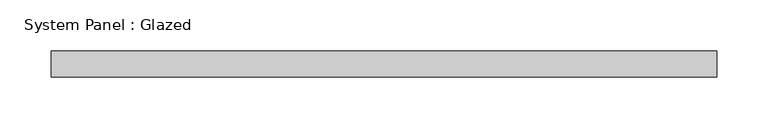
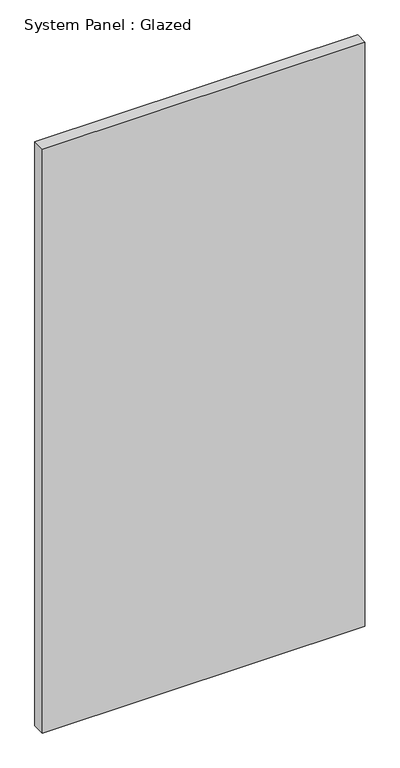
"""IFC4 building model written with IfcOpenShell, lengths in millimetres: plate geometry, System Panel : Glazed."""

from ifc_helpers import new_model, si_unit, origin, origin_with_axes, place, context, project, spatial, polyline, outline, extrude, source, transform, mapped, element, save


def system_panel_glazed_1f6aae05(model_context):
    return source(origin(), model_context, "Body", "SweptSolid", [
        extrude(outline(polyline([(323.85, 19.05), (-323.85, 19.05), (-323.85, 44.45), (323.85, 44.45), (323.85, 19.05)])), origin_with_axes(), (0.0, 0.0, 1.0), 1239.313455),
    ])


if __name__ == "__main__":
    model = new_model("IFC4")
    model_context = context("Model", 3, world=origin())
    ifc_project = project(units=[si_unit("LENGTHUNIT", "METRE", prefix="MILLI")], contexts=[model_context])
    site = spatial("IfcSite", under=ifc_project)
    building = spatial("IfcBuilding", under=site)
    placement = place(None, origin())
    system_panel_glazed_shape = system_panel_glazed_1f6aae05(model_context)
    element("IfcPlate", 1, ObjectType="System Panel : Glazed", at=placement, inside=building, context=model_context, shape_type="MappedRepresentation", body=[
        mapped(system_panel_glazed_shape, transform((0.0, 0.0, 0.0), x_axis=(1.0, 0.0, 0.0), y_axis=(0.0, 1.0, 0.0), z_axis=(0.0, 0.0, 1.0))),
    ])
    save(model, "model.ifc")

# Revit data of these elements
# Type "System Panel : Glazed"
#   Construction Type Id = "GSP4R"
#   Analytic Construction = "1/8 in Pilkington single glazing"
#   Visual Light Transmittance = 0.9
#   Solar Heat Gain Coefficient = 0.86
#   Heat Transfer Coefficient (U) = 1.18115 BTU/(h·ft²·°F)
#   Define Thermal Properties by = 1
# Element 1 (IfcPlate, "System Panel : Glazed")
#   Materials on its faces: "Glass"
# Materials
#   "Glass": class "Glass", colour RGB 0 128 192, transparency 0.75, Description = "Soda Lime Glass", Cost = 0
